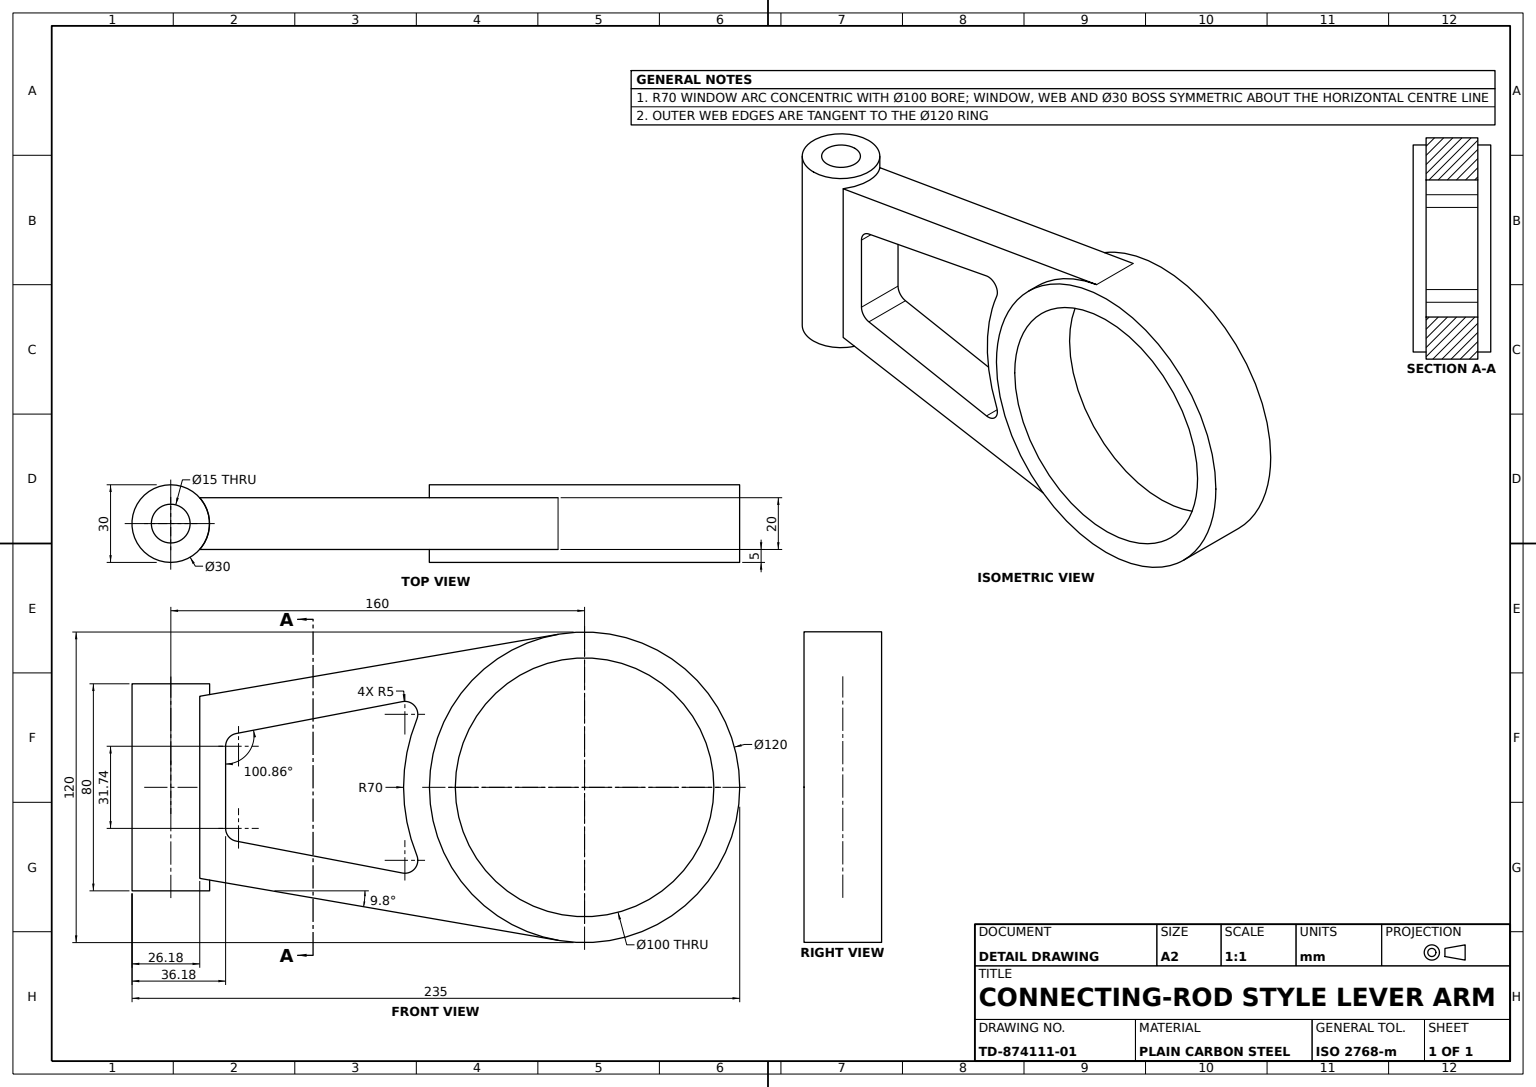
from build123d import *

# Parameters (mm, degrees)
BIG_END_RING_SKETCH_R       = 60
BIG_END_RING_SKETCH_R_2     = 50
BIG_END_RING_120_DEPTH      = 15
SMALL_END_BOSS_SKETCH_R     = 15
SMALL_END_BOSS_SKETCH_R_2   = 7.5
SMALL_END_BOSS_30_DEPTH     = 40
CONNECTING_WEB_DEPTH        = 10
WEB_LIGHTENING_WINDOW_DEPTH = 52.5


with BuildPart() as part:
    # Big End Ring Sketch → Big End Ring Ø120 (new, symmetric)
    with BuildSketch(Plane.XY):
        Circle(BIG_END_RING_SKETCH_R)
        Circle(BIG_END_RING_SKETCH_R_2, mode=Mode.SUBTRACT)
    extrude(amount=BIG_END_RING_120_DEPTH, both=True)



with BuildPart() as body_2:
    # Small End Boss Sketch → Small End Boss Ø30 (new, symmetric)
    with BuildSketch(Plane(origin=(0, 0, 0), x_dir=(1, 0, 0), z_dir=(0, 1, 0))):
        with Locations(Location((-160, 0, 0), (0, 0, 270))):
            Circle(SMALL_END_BOSS_SKETCH_R)
        with Locations(Location((-160, 0, 0), (0, 0, 270))):
            Circle(SMALL_END_BOSS_SKETCH_R_2, mode=Mode.SUBTRACT)
    extrude(amount=SMALL_END_BOSS_30_DEPTH, both=True)


with BuildPart() as part_1:
    add(part.part)

    add(body_2.part)  # Connecting Web merges body 2
    # Web Profile Sketch → Connecting Web (add, symmetric)
    with BuildSketch(Plane.XY):
        with BuildLine():
            Line((-10.212938139, 59.12441031), (-149.873192049, 35))
            Line((-149.873192049, 35), (-149.873192049, -35))
            Line((-149.873192049, -35), (-10.212938139, -59.12441031))
            ThreePointArc((-10.212938139, -59.12441031), (-60, 0), (-10.212938139, 59.12441031))
        make_face()
    extrude(amount=CONNECTING_WEB_DEPTH, both=True)

    # Web Window Sketch → Web Lightening Window (cut, symmetric)
    with BuildSketch(Plane.XY.offset(10)):
        with BuildLine():
            Line((-138.819660113, 15.867947938), (-138.819660113, -15.867947938))
            ThreePointArc((-138.819660113, -15.867947938), (-137.673856674, -19.053096108), (-134.761592567, -20.778422788))
            Line((-134.761592567, -20.778422788), (-70.43555138, -33.117511712))
            ThreePointArc((-70.43555138, -33.117511712), (-65.629029038, -31.379566609), (-64.860710998, -26.326567738))
            ThreePointArc((-64.860710998, -26.326567738), (-70, 0), (-64.860710998, 26.326567738))
            ThreePointArc((-64.860710998, 26.326567738), (-65.629029038, 31.379566609), (-70.43555138, 33.117511712))
            Line((-70.43555138, 33.117511712), (-134.761592567, 20.778422788))
            ThreePointArc((-134.761592567, 20.778422788), (-137.673856674, 19.053096108), (-138.819660113, 15.867947938))
        make_face()
    extrude(amount=WEB_LIGHTENING_WINDOW_DEPTH, both=True, mode=Mode.SUBTRACT)


solid = part_1.part
